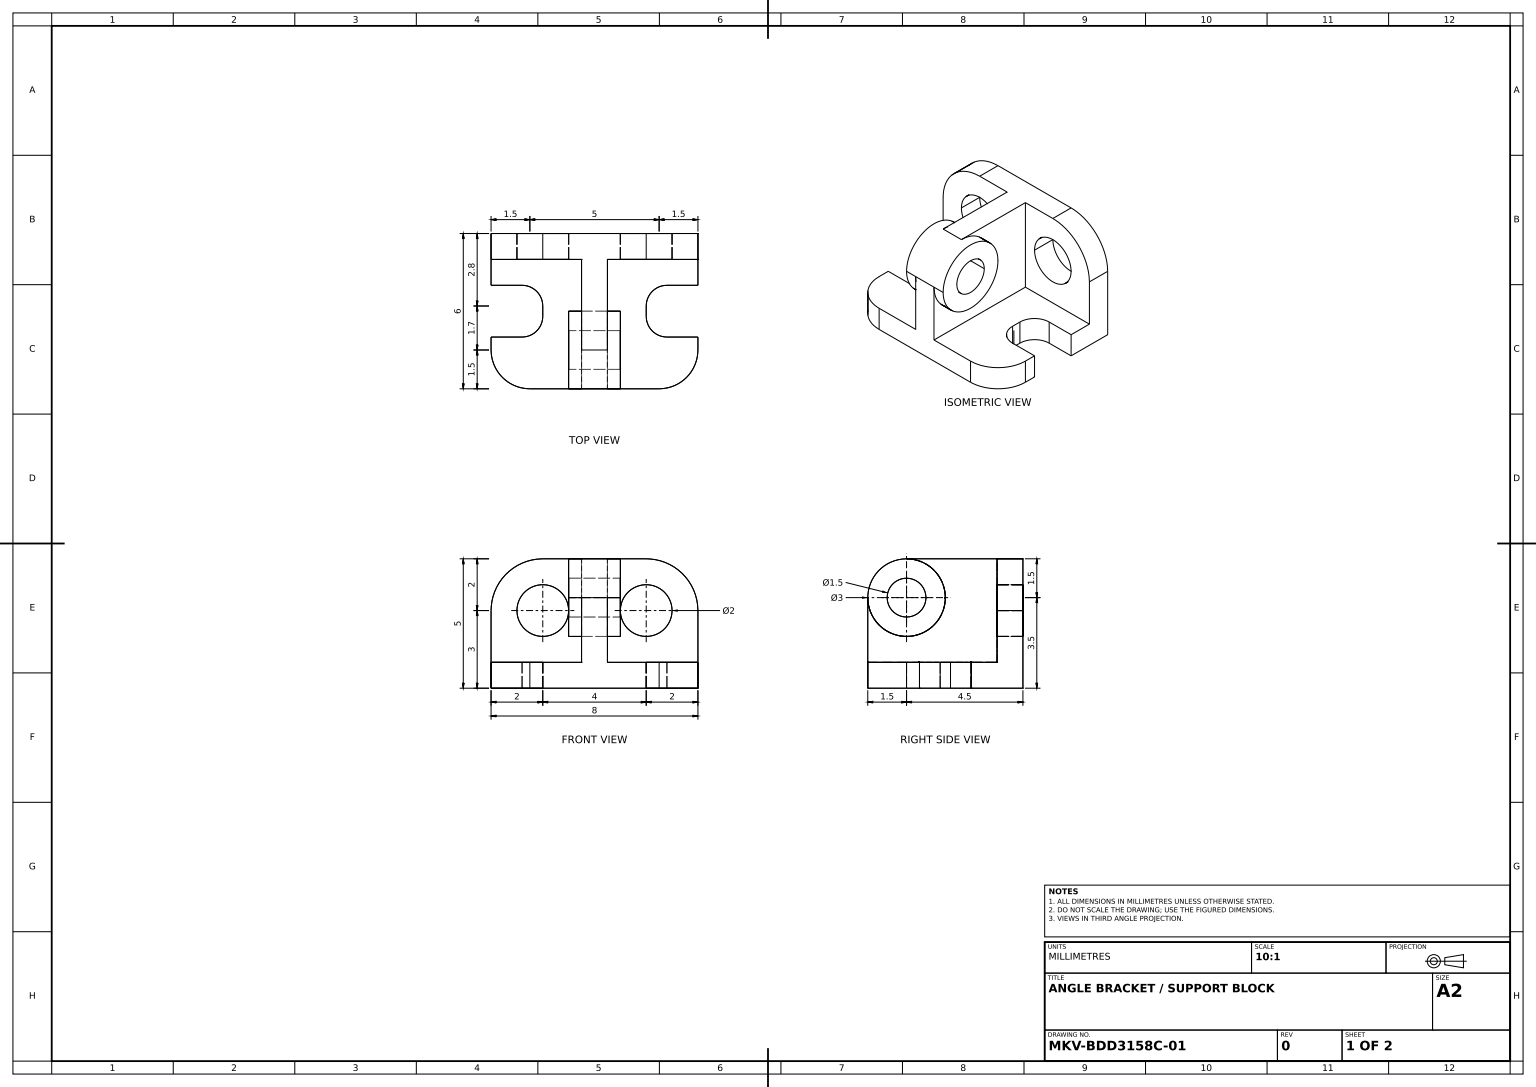
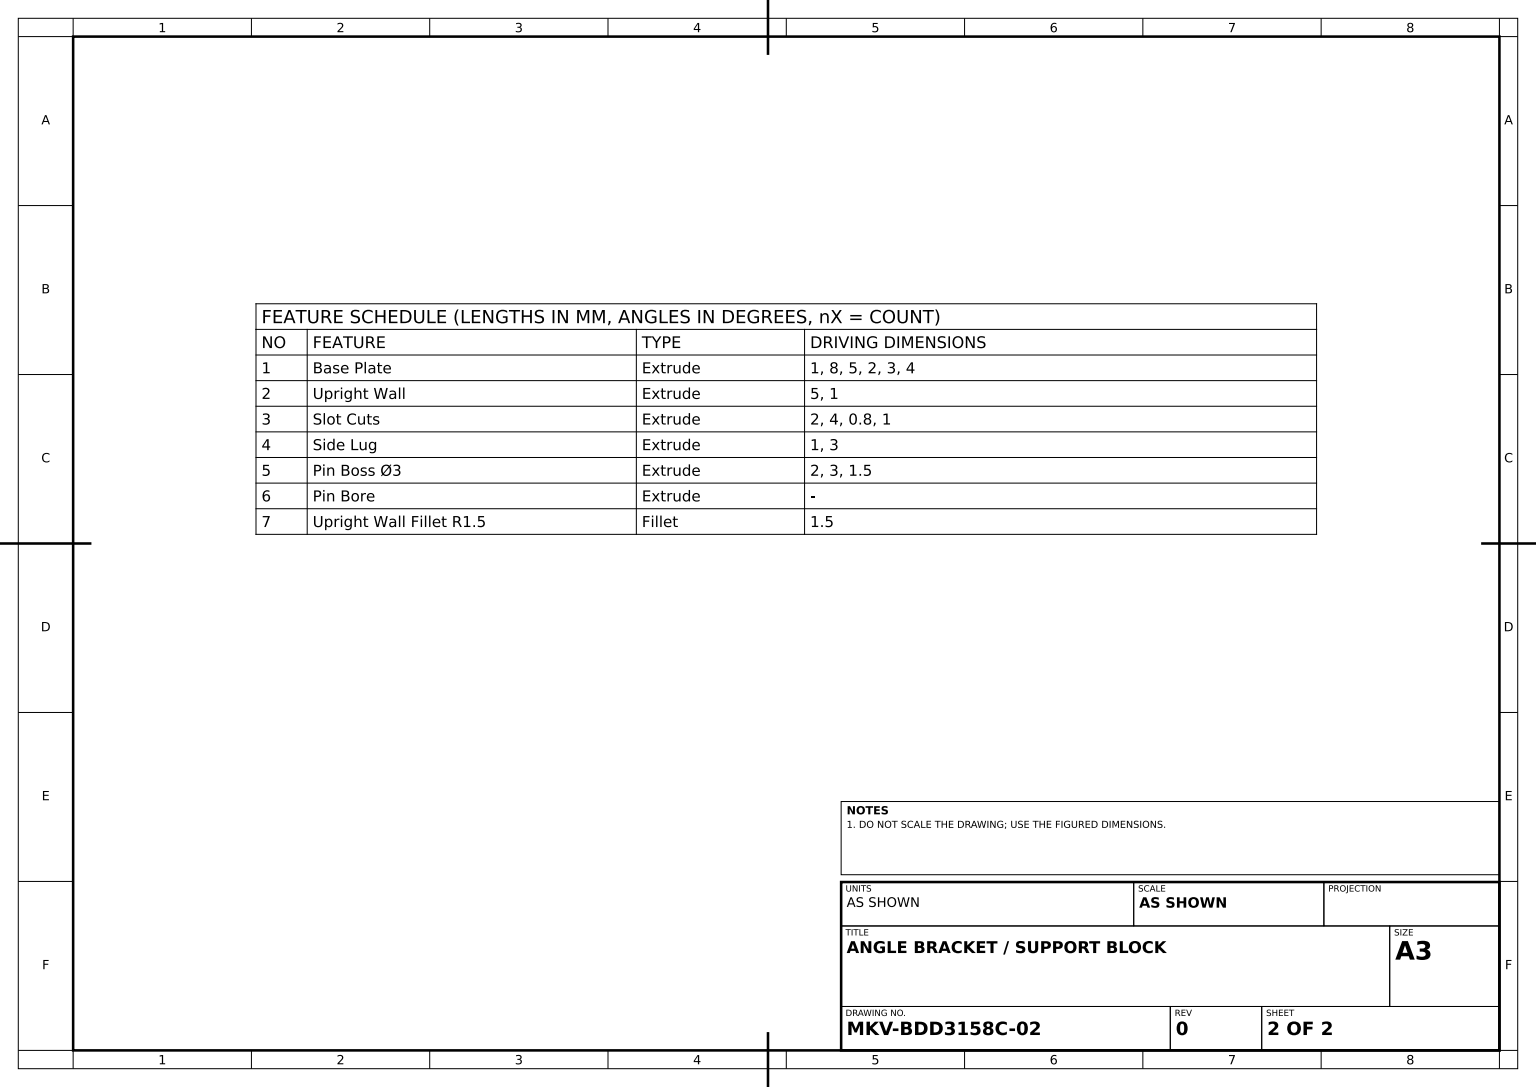
from build123d import *

# Parameters (mm, degrees)
BASE_PLATE_SKETCH_R        = 1
BASE_PLATE_DEPTH           = 1
UPRIGHT_WALL_SKETCH_W      = 8
UPRIGHT_WALL_SKETCH_H      = 1
UPRIGHT_WALL_DEPTH         = 5
SLOT_CUTS_DEPTH            = 9.246211251
SIDE_LUG_DEPTH             = 0.5
PIN_BOSS_SKETCH_R          = 1.5
PIN_BOSS_SKETCH_R_2        = 0.75
PIN_BOSS_3_DEPTH           = 1
PIN_BORE_SKETCH_R          = 0.75
PIN_BORE_DEPTH             = 8.90569415
UPRIGHT_WALL_FILLET_R1_5_R = 1.5


with BuildPart() as part:
    # Base Plate Sketch → Base Plate (new body)
    with BuildSketch(Plane.XY):
        with BuildLine():
            Line((-2, 2.5), (2, 2.5))
            ThreePointArc((2, 2.5), (3.414213562, 1.914213562), (4, 0.5))
            Line((4, 0.5), (4, -2.5))
            Line((4, -2.5), (-4, -2.5))
            Line((-4, -2.5), (-4, 0.5))
            ThreePointArc((-4, 0.5), (-3.414213562, 1.914213562), (-2, 2.5))
        make_face()
        with Locations((-2, 0.5)):
            Circle(BASE_PLATE_SKETCH_R, mode=Mode.SUBTRACT)
        with Locations((2, 0.5)):
            Circle(BASE_PLATE_SKETCH_R, mode=Mode.SUBTRACT)
    extrude(amount=BASE_PLATE_DEPTH)

    # Upright Wall Sketch → Upright Wall (add)
    with BuildSketch(Plane.XY.offset(1)):
        with Locations((0, -2)):
            Rectangle(UPRIGHT_WALL_SKETCH_W, UPRIGHT_WALL_SKETCH_H)
    extrude(amount=UPRIGHT_WALL_DEPTH)

    # Slot Cuts Sketch → Slot Cuts (cut, through all)
    with BuildSketch(Plane(origin=(0, -1.5, 0), x_dir=(1, 0, 0), z_dir=(0, 1, 0))):
        with BuildLine():
            Line((-4, -2), (-2.8, -2))
            ThreePointArc((-2.8, -2), (-2.234314575, -2.234314575), (-2, -2.8))
            Line((-2, -2.8), (-2, -3.2))
            ThreePointArc((-2, -3.2), (-2.234314575, -3.765685425), (-2.8, -4))
            Line((-2.8, -4), (-4, -4))
            Line((-4, -4), (-4, -2))
        make_face()
        with BuildLine():
            Line((4, -2), (2.8, -2))
            ThreePointArc((2.8, -2), (2.234314575, -2.234314575), (2, -2.8))
            Line((2, -2.8), (2, -3.2))
            ThreePointArc((2, -3.2), (2.234314575, -3.765685425), (2.8, -4))
            Line((2.8, -4), (4, -4))
            Line((4, -4), (4, -2))
        make_face()
    extrude(amount=-SLOT_CUTS_DEPTH, mode=Mode.SUBTRACT)

    # Side Lug Sketch → Side Lug (add, symmetric)
    with BuildSketch(Plane(origin=(0, 0, 0), x_dir=(0, 0, -1), z_dir=(1, 0, 0))):
        with BuildLine():
            Line((-1, 2.5), (-4.5, 2.5))
            ThreePointArc((-4.5, 2.5), (-5.560660172, 2.060660172), (-6, 1))
            Line((-6, 1), (-6, -1.5))
            Line((-6, -1.5), (-1, -1.5))
            Line((-1, -1.5), (-1, 2.5))
        make_face()
    extrude(amount=SIDE_LUG_DEPTH, both=True)

    # Pin Boss Sketch → Pin Boss Ø3 (add, symmetric)
    with BuildSketch(Plane(origin=(0, 0, 0), x_dir=(0, 0, -1), z_dir=(1, 0, 0))):
        with Locations((-4.5, 1)):
            Circle(PIN_BOSS_SKETCH_R)
        with Locations((-4.5, 1)):
            Circle(PIN_BOSS_SKETCH_R_2, mode=Mode.SUBTRACT)
    extrude(amount=PIN_BOSS_3_DEPTH, both=True)

    # Pin Bore Sketch → Pin Bore (cut, through all)
    with BuildSketch(Plane(origin=(0.5, 0, 0), x_dir=(0, 0, -1), z_dir=(1, 0, 0))):
        with Locations((-4.5, 1)):
            Circle(PIN_BORE_SKETCH_R)
    extrude(amount=-PIN_BORE_DEPTH, mode=Mode.SUBTRACT)

    # Upright Wall Fillet R1.5
    upright_wall_fillet_r1_5_edges = [part.edges().sort_by_distance(p)[0] for p in [
        (-4, -2, 6),
        (4, -2, 6),
    ]]
    fillet(upright_wall_fillet_r1_5_edges, radius=UPRIGHT_WALL_FILLET_R1_5_R)


solid = part.part
